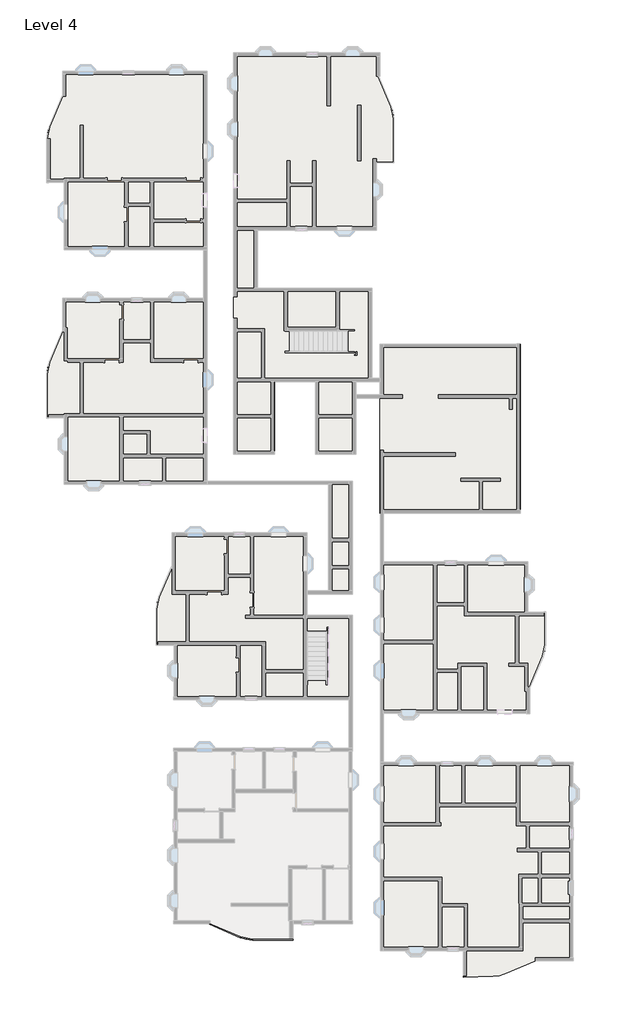
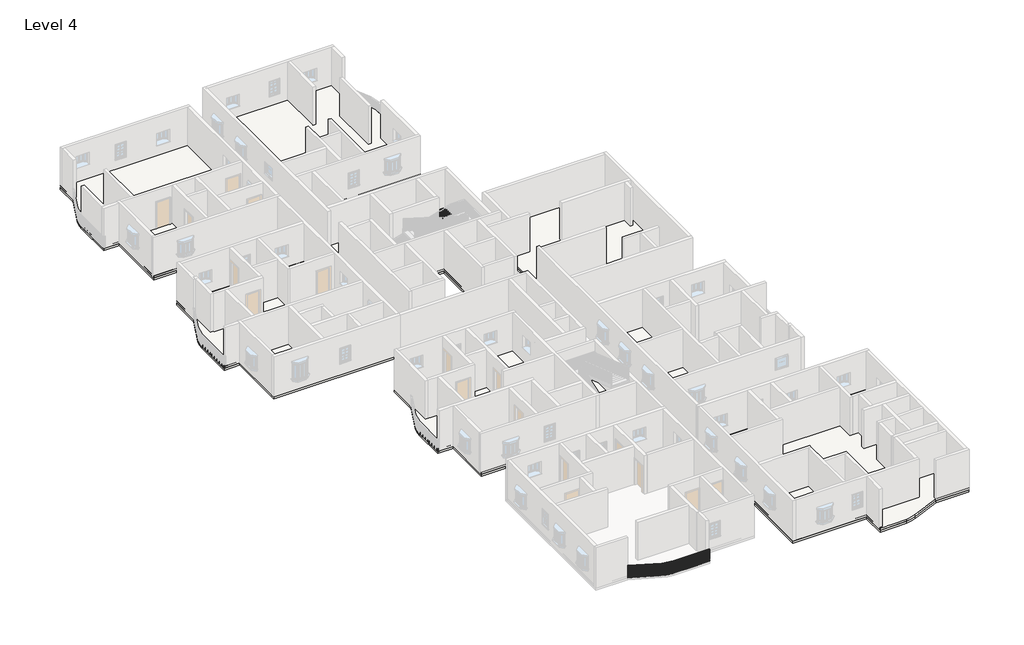
# One storey, part 5 of 14: 13 roofs, 12 slabs, 1 railing.
"""IFC4 building model written with IfcOpenShell, lengths in millimetres."""

from ifc_helpers import new_model, si_unit, point, frame, frame_2d, origin, place, context, project, spatial, polyline, circle_curve, trimmed, segment, composite_curve, outline, extrude, element, save
from ifc_brep_helpers import plane_surface, cylinder_surface, revolved_surface, advanced_brep

model = new_model("IFC4")

# Units and contexts
model_context = context("Model", 3, world=origin())
ifc_project = project(units=[si_unit("LENGTHUNIT", "METRE", prefix="MILLI")], contexts=[model_context])

# Site, building, storey
site = spatial("IfcSite", under=ifc_project)
building = spatial("IfcBuilding", under=site)
storey = spatial("IfcBuildingStorey", under=building, Name="Level 4", Elevation=9144.0)

# Railing
placement = place(None, origin())
element("IfcRailing", 1, ObjectType="Handrail - Rectangular", at=placement, inside=storey, context=model_context, shape_type="SolidModel", body=[
    advanced_brep(
    [(-10014.8722294, -25076.9923935, 10058.4), (-10014.8722294, -25076.9923935, 10007.6), (-10034.8694485, -25123.6909077, 10007.6), (-10034.8694485, -25123.6909077, 10058.4), (-8065.5370278, -25911.7359335, 10058.4), (-8065.5370278, -25911.7359335, 10007.6), (-8085.5342469, -25958.4344477, 10007.6), (-8085.5342469, -25958.4344477, 10058.4), (-7315.6413127, -26065.5416506, 10007.6), (-7315.6413127, -26065.5416506, 10058.4), (-7315.6413127, -26116.3416506, 10007.6), (-7315.6413127, -26116.3416506, 10058.4), (-4746.0891351, -26065.5416506, 10058.4), (-4746.0891351, -26116.3416506, 10058.4), (-4746.0891351, -26116.3416506, 10007.6), (-4746.0891351, -26065.5416506, 10007.6)],
    [
        (0, 1),
        (1, 2),
        (2, 3),
        (3, 0),
        (0, 4),
        (4, 5),
        (5, 1),
        (5, 6),
        (6, 2),
        (6, 7),
        (7, 3),
        (7, 4),
        (8, 5, circle_curve(frame((-7315.6413127, -24160.5416506, 10007.6), z_axis=(0.0, 0.0, -1.0), x_axis=(-0.3936460446736572, -0.9192620907623599, 0.0)), 1905.0)),
        (4, 9, circle_curve(frame((-7315.6413127, -24160.5416506, 10058.4), z_axis=(0.0, 0.0, 1.0), x_axis=(-0.3936460446736572, -0.9192620907623599, 0.0)), 1905.0)),
        (9, 8),
        (10, 6, circle_curve(frame((-7315.6413127, -24160.5416506, 10007.6), z_axis=(0.0, 0.0, -1.0), x_axis=(-0.3936460446736572, -0.9192620907623599, 0.0)), 1955.8)),
        (8, 10),
        (11, 7, circle_curve(frame((-7315.6413127, -24160.5416506, 10058.4), z_axis=(0.0, 0.0, -1.0), x_axis=(-0.3936460446736572, -0.9192620907623599, 0.0)), 1955.8)),
        (10, 11),
        (11, 9),
        (12, 13),
        (13, 14),
        (14, 15),
        (15, 12),
        (9, 12),
        (15, 8),
        (14, 10),
        (13, 11),
    ],
    [
        plane_surface(frame((-10024.8708389, -25100.3416506, 10058.4), z_axis=(-0.9192620907623597, 0.39364604467365766, 0.0), x_axis=(0.39364604467365766, 0.9192620907623597, 0.0))),
        plane_surface(frame((-10014.8722294, -25076.9923935, 10058.4), z_axis=(0.3936460446736573, 0.9192620907623599, 0.0), x_axis=(0.9192620907623599, -0.3936460446736573, 0.0))),
        plane_surface(frame((-10014.8722294, -25076.9923935, 10007.6), z_axis=(0.0, 0.0, -1.0000000000000002), x_axis=(0.9192620907623599, -0.3936460446736573, 0.0))),
        plane_surface(frame((-10034.8694485, -25123.6909077, 10007.6), z_axis=(-0.39364604467365766, -0.9192620907623597, 0.0), x_axis=(0.9192620907623597, -0.39364604467365766, 0.0))),
        plane_surface(frame((-10034.8694485, -25123.6909077, 10058.4), z_axis=(0.0, 0.0, 1.0), x_axis=(0.9192620907623597, -0.39364604467365766, 0.0))),
        revolved_surface(polyline([(-8065.537027803317, -25911.735933502296, 10058.4), (-8065.537027803317, -25911.735933502296, 10007.6)]), (-7315.6413127, -24160.5416506, 10058.4), (0.0, 0.0, 1.0)),
        plane_surface(frame((-7315.6413127, -24160.5416506, 10007.6), z_axis=(0.0, 0.0, -1.0), x_axis=(-0.3936460446736572, -0.9192620907623599, 0.0))),
        cylinder_surface(frame((-7315.6413127, -24160.5416506, 10058.4), z_axis=(0.0, 0.0, 1.0), x_axis=(-0.3936460446736572, -0.9192620907623599, 0.0)), 1955.8),
        plane_surface(frame((-7315.6413127, -24160.5416506, 10058.4), z_axis=(0.0, 0.0, 1.0), x_axis=(-0.3936460446736572, -0.9192620907623599, 0.0))),
        plane_surface(frame((-4746.0891351, -26090.9416506, 10058.4), z_axis=(1.0, 0.0, 0.0), x_axis=(0.0, 1.0, 0.0))),
        plane_surface(frame((-7315.6413127, -26065.5416506, 10058.4), z_axis=(0.0, 1.0, 0.0), x_axis=(1.0, 0.0, 0.0))),
        plane_surface(frame((-7315.6413127, -26065.5416506, 10007.6), z_axis=(0.0, 0.0, -1.0), x_axis=(1.0, 0.0, 0.0))),
        plane_surface(frame((-7315.6413127, -26116.3416506, 10007.6), z_axis=(0.0, -1.0, 0.0), x_axis=(1.0, 0.0, 0.0))),
        plane_surface(frame((-7315.6413127, -26116.3416506, 10058.4), z_axis=(0.0, 0.0, 1.0), x_axis=(1.0, 0.0, 0.0))),
    ],
    [
        (0, [[1, 2, 3, 4]]),
        (1, [[-1, 5, 6, 7]]),
        (2, [[-2, -7, 8, 9]]),
        (3, [[-3, -9, 10, 11]]),
        (4, [[-4, -11, 12, -5]]),
        (5, [[13, -6, 14, 15]]),
        (6, [[16, -8, -13, 17]]),
        (7, [[18, -10, -16, 19]]),
        (8, [[-14, -12, -18, 20]]),
        (9, [[21, 22, 23, 24]]),
        (10, [[-15, 25, -24, 26]]),
        (11, [[-17, -26, -23, 27]]),
        (12, [[-19, -27, -22, 28]]),
        (13, [[-20, -28, -21, -25]]),
    ],
),
    extrude(outline(polyline([(-4785.1663127, -26100.4666506), (-4785.1663127, -26081.4166506), (-4766.1163127, -26081.4166506), (-4766.1163127, -26100.4666506), (-4785.1663127, -26100.4666506)])), frame((0.0, 0.0, 9144.0), z_axis=(0.0, 0.0, 1.0), x_axis=(1.0, 0.0, 0.0)), (0.0, 0.0, 1.0), 863.6),
    extrude(outline(polyline([(-4886.7663127, -26100.4666506), (-4886.7663127, -26081.4166506), (-4867.7163127, -26081.4166506), (-4867.7163127, -26100.4666506), (-4886.7663127, -26100.4666506)])), frame((0.0, 0.0, 9144.0), z_axis=(0.0, 0.0, 1.0), x_axis=(1.0, 0.0, 0.0)), (0.0, 0.0, 1.0), 863.6),
    extrude(outline(polyline([(-4988.3663127, -26100.4666506), (-4988.3663127, -26081.4166506), (-4969.3163127, -26081.4166506), (-4969.3163127, -26100.4666506), (-4988.3663127, -26100.4666506)])), frame((0.0, 0.0, 9144.0), z_axis=(0.0, 0.0, 1.0), x_axis=(1.0, 0.0, 0.0)), (0.0, 0.0, 1.0), 863.6),
    extrude(outline(polyline([(-5089.9663127, -26100.4666506), (-5089.9663127, -26081.4166506), (-5070.9163127, -26081.4166506), (-5070.9163127, -26100.4666506), (-5089.9663127, -26100.4666506)])), frame((0.0, 0.0, 9144.0), z_axis=(0.0, 0.0, 1.0), x_axis=(1.0, 0.0, 0.0)), (0.0, 0.0, 1.0), 863.6),
    extrude(outline(polyline([(-5191.5663127, -26100.4666506), (-5191.5663127, -26081.4166506), (-5172.5163127, -26081.4166506), (-5172.5163127, -26100.4666506), (-5191.5663127, -26100.4666506)])), frame((0.0, 0.0, 9144.0), z_axis=(0.0, 0.0, 1.0), x_axis=(1.0, 0.0, 0.0)), (0.0, 0.0, 1.0), 863.6),
    extrude(outline(polyline([(-5293.1663127, -26100.4666506), (-5293.1663127, -26081.4166506), (-5274.1163127, -26081.4166506), (-5274.1163127, -26100.4666506), (-5293.1663127, -26100.4666506)])), frame((0.0, 0.0, 9144.0), z_axis=(0.0, 0.0, 1.0), x_axis=(1.0, 0.0, 0.0)), (0.0, 0.0, 1.0), 863.6),
    extrude(outline(polyline([(-5394.7663127, -26100.4666506), (-5394.7663127, -26081.4166506), (-5375.7163127, -26081.4166506), (-5375.7163127, -26100.4666506), (-5394.7663127, -26100.4666506)])), frame((0.0, 0.0, 9144.0), z_axis=(0.0, 0.0, 1.0), x_axis=(1.0, 0.0, 0.0)), (0.0, 0.0, 1.0), 863.6),
    extrude(outline(polyline([(-5496.3663127, -26100.4666506), (-5496.3663127, -26081.4166506), (-5477.3163127, -26081.4166506), (-5477.3163127, -26100.4666506), (-5496.3663127, -26100.4666506)])), frame((0.0, 0.0, 9144.0), z_axis=(0.0, 0.0, 1.0), x_axis=(1.0, 0.0, 0.0)), (0.0, 0.0, 1.0), 863.6),
    extrude(outline(polyline([(-5597.9663127, -26100.4666506), (-5597.9663127, -26081.4166506), (-5578.9163127, -26081.4166506), (-5578.9163127, -26100.4666506), (-5597.9663127, -26100.4666506)])), frame((0.0, 0.0, 9144.0), z_axis=(0.0, 0.0, 1.0), x_axis=(1.0, 0.0, 0.0)), (0.0, 0.0, 1.0), 863.6),
    extrude(outline(polyline([(-5699.5663127, -26100.4666506), (-5699.5663127, -26081.4166506), (-5680.5163127, -26081.4166506), (-5680.5163127, -26100.4666506), (-5699.5663127, -26100.4666506)])), frame((0.0, 0.0, 9144.0), z_axis=(0.0, 0.0, 1.0), x_axis=(1.0, 0.0, 0.0)), (0.0, 0.0, 1.0), 863.6),
    extrude(outline(polyline([(-5801.1663127, -26100.4666506), (-5801.1663127, -26081.4166506), (-5782.1163127, -26081.4166506), (-5782.1163127, -26100.4666506), (-5801.1663127, -26100.4666506)])), frame((0.0, 0.0, 9144.0), z_axis=(0.0, 0.0, 1.0), x_axis=(1.0, 0.0, 0.0)), (0.0, 0.0, 1.0), 863.6),
    extrude(outline(polyline([(-5902.7663127, -26100.4666506), (-5902.7663127, -26081.4166506), (-5883.7163127, -26081.4166506), (-5883.7163127, -26100.4666506), (-5902.7663127, -26100.4666506)])), frame((0.0, 0.0, 9144.0), z_axis=(0.0, 0.0, 1.0), x_axis=(1.0, 0.0, 0.0)), (0.0, 0.0, 1.0), 863.6),
    extrude(outline(polyline([(-6004.3663127, -26100.4666506), (-6004.3663127, -26081.4166506), (-5985.3163127, -26081.4166506), (-5985.3163127, -26100.4666506), (-6004.3663127, -26100.4666506)])), frame((0.0, 0.0, 9144.0), z_axis=(0.0, 0.0, 1.0), x_axis=(1.0, 0.0, 0.0)), (0.0, 0.0, 1.0), 863.6),
    extrude(outline(polyline([(-6105.9663127, -26100.4666506), (-6105.9663127, -26081.4166506), (-6086.9163127, -26081.4166506), (-6086.9163127, -26100.4666506), (-6105.9663127, -26100.4666506)])), frame((0.0, 0.0, 9144.0), z_axis=(0.0, 0.0, 1.0), x_axis=(1.0, 0.0, 0.0)), (0.0, 0.0, 1.0), 863.6),
    extrude(outline(polyline([(-6207.5663127, -26100.4666506), (-6207.5663127, -26081.4166506), (-6188.5163127, -26081.4166506), (-6188.5163127, -26100.4666506), (-6207.5663127, -26100.4666506)])), frame((0.0, 0.0, 9144.0), z_axis=(0.0, 0.0, 1.0), x_axis=(1.0, 0.0, 0.0)), (0.0, 0.0, 1.0), 863.6),
    extrude(outline(polyline([(-6309.1663127, -26100.4666506), (-6309.1663127, -26081.4166506), (-6290.1163127, -26081.4166506), (-6290.1163127, -26100.4666506), (-6309.1663127, -26100.4666506)])), frame((0.0, 0.0, 9144.0), z_axis=(0.0, 0.0, 1.0), x_axis=(1.0, 0.0, 0.0)), (0.0, 0.0, 1.0), 863.6),
    extrude(outline(polyline([(-6410.7663127, -26100.4666506), (-6410.7663127, -26081.4166506), (-6391.7163127, -26081.4166506), (-6391.7163127, -26100.4666506), (-6410.7663127, -26100.4666506)])), frame((0.0, 0.0, 9144.0), z_axis=(0.0, 0.0, 1.0), x_axis=(1.0, 0.0, 0.0)), (0.0, 0.0, 1.0), 863.6),
    extrude(outline(polyline([(-6512.3663127, -26100.4666506), (-6512.3663127, -26081.4166506), (-6493.3163127, -26081.4166506), (-6493.3163127, -26100.4666506), (-6512.3663127, -26100.4666506)])), frame((0.0, 0.0, 9144.0), z_axis=(0.0, 0.0, 1.0), x_axis=(1.0, 0.0, 0.0)), (0.0, 0.0, 1.0), 863.6),
    extrude(outline(polyline([(-6613.9663127, -26100.4666506), (-6613.9663127, -26081.4166506), (-6594.9163127, -26081.4166506), (-6594.9163127, -26100.4666506), (-6613.9663127, -26100.4666506)])), frame((0.0, 0.0, 9144.0), z_axis=(0.0, 0.0, 1.0), x_axis=(1.0, 0.0, 0.0)), (0.0, 0.0, 1.0), 863.6),
    extrude(outline(polyline([(-6715.5663127, -26100.4666506), (-6715.5663127, -26081.4166506), (-6696.5163127, -26081.4166506), (-6696.5163127, -26100.4666506), (-6715.5663127, -26100.4666506)])), frame((0.0, 0.0, 9144.0), z_axis=(0.0, 0.0, 1.0), x_axis=(1.0, 0.0, 0.0)), (0.0, 0.0, 1.0), 863.6),
    extrude(outline(polyline([(-6817.1663127, -26100.4666506), (-6817.1663127, -26081.4166506), (-6798.1163127, -26081.4166506), (-6798.1163127, -26100.4666506), (-6817.1663127, -26100.4666506)])), frame((0.0, 0.0, 9144.0), z_axis=(0.0, 0.0, 1.0), x_axis=(1.0, 0.0, 0.0)), (0.0, 0.0, 1.0), 863.6),
    extrude(outline(polyline([(-6918.7663127, -26100.4666506), (-6918.7663127, -26081.4166506), (-6899.7163127, -26081.4166506), (-6899.7163127, -26100.4666506), (-6918.7663127, -26100.4666506)])), frame((0.0, 0.0, 9144.0), z_axis=(0.0, 0.0, 1.0), x_axis=(1.0, 0.0, 0.0)), (0.0, 0.0, 1.0), 863.6),
    extrude(outline(polyline([(-7020.3663127, -26100.4666506), (-7020.3663127, -26081.4166506), (-7001.3163127, -26081.4166506), (-7001.3163127, -26100.4666506), (-7020.3663127, -26100.4666506)])), frame((0.0, 0.0, 9144.0), z_axis=(0.0, 0.0, 1.0), x_axis=(1.0, 0.0, 0.0)), (0.0, 0.0, 1.0), 863.6),
    extrude(outline(polyline([(-7121.9663127, -26100.4666506), (-7121.9663127, -26081.4166506), (-7102.9163127, -26081.4166506), (-7102.9163127, -26100.4666506), (-7121.9663127, -26100.4666506)])), frame((0.0, 0.0, 9144.0), z_axis=(0.0, 0.0, 1.0), x_axis=(1.0, 0.0, 0.0)), (0.0, 0.0, 1.0), 863.6),
    extrude(outline(polyline([(-7223.5663127, -26100.4666506), (-7223.5663127, -26081.4166506), (-7204.5163127, -26081.4166506), (-7204.5163127, -26100.4666506), (-7223.5663127, -26100.4666506)])), frame((0.0, 0.0, 9144.0), z_axis=(0.0, 0.0, 1.0), x_axis=(1.0, 0.0, 0.0)), (0.0, 0.0, 1.0), 863.6),
    extrude(outline(polyline([(-7395.3185803, -26098.8530973), (-7394.6296262, -26079.8155596), (-7375.5920885, -26080.5045137), (-7376.2810426, -26099.5420514), (-7395.3185803, -26098.8530973)])), frame((0.0, 0.0, 9144.0), z_axis=(0.0, 0.0, 1.0), x_axis=(1.0, 0.0, 0.0)), (0.0, 0.0, 1.0), 863.6),
    extrude(outline(polyline([(-7497.177549, -26091.9774704), (-7495.4880357, -26073.0025384), (-7476.5131037, -26074.6920517), (-7478.2026169, -26093.6669837), (-7497.177549, -26091.9774704)])), frame((0.0, 0.0, 9144.0), z_axis=(0.0, 0.0, 1.0), x_axis=(1.0, 0.0, 0.0)), (0.0, 0.0, 1.0), 863.6),
    extrude(outline(polyline([(-7598.5337632, -26079.7528408), (-7595.8483698, -26060.8930645), (-7576.9885935, -26063.5784579), (-7579.6739869, -26082.4382342), (-7598.5337632, -26079.7528408)])), frame((0.0, 0.0, 9144.0), z_axis=(0.0, 0.0, 1.0), x_axis=(1.0, 0.0, 0.0)), (0.0, 0.0, 1.0), 863.6),
    extrude(outline(polyline([(-7699.1065227, -26062.2130639), (-7695.4326862, -26043.5206744), (-7676.7402967, -26047.1945108), (-7680.4141332, -26065.8869003), (-7699.1065227, -26062.2130639)])), frame((0.0, 0.0, 9144.0), z_axis=(0.0, 0.0, 1.0), x_axis=(1.0, 0.0, 0.0)), (0.0, 0.0, 1.0), 863.6),
    extrude(outline(polyline([(-7798.6172969, -26039.4067149), (-7793.9651918, -26020.9334797), (-7775.4919566, -26025.5855848), (-7780.1440617, -26044.05882), (-7798.6172969, -26039.4067149)])), frame((0.0, 0.0, 9144.0), z_axis=(0.0, 0.0, 1.0), x_axis=(1.0, 0.0, 0.0)), (0.0, 0.0, 1.0), 863.6),
    extrude(outline(polyline([(-7896.7904963, -26011.396955), (-7891.1730064, -25993.1940347), (-7872.9700861, -25998.8115246), (-7878.587576, -26017.0144449), (-7896.7904963, -26011.396955)])), frame((0.0, 0.0, 9144.0), z_axis=(0.0, 0.0, 1.0), x_axis=(1.0, 0.0, 0.0)), (0.0, 0.0, 1.0), 863.6),
    extrude(outline(polyline([(-7993.3542357, -25978.2613554), (-7986.7869183, -25960.379162), (-7968.9047249, -25966.9464794), (-7975.4720423, -25984.8286729), (-7993.3542357, -25978.2613554)])), frame((0.0, 0.0, 9144.0), z_axis=(0.0, 0.0, 1.0), x_axis=(1.0, 0.0, 0.0)), (0.0, 0.0, 1.0), 863.6),
    extrude(outline(polyline([(-8169.4357205, -25905.2369062), (-8161.9367633, -25887.7249634), (-8144.4248205, -25895.2239205), (-8151.9237777, -25912.7358634), (-8169.4357205, -25905.2369062)])), frame((0.0, 0.0, 9144.0), z_axis=(0.0, 0.0, 1.0), x_axis=(1.0, 0.0, 0.0)), (0.0, 0.0, 1.0), 863.6),
    extrude(outline(polyline([(-8262.8327489, -25865.2424681), (-8255.3337918, -25847.7305252), (-8237.8218489, -25855.2294824), (-8245.3208061, -25872.7414252), (-8262.8327489, -25865.2424681)])), frame((0.0, 0.0, 9144.0), z_axis=(0.0, 0.0, 1.0), x_axis=(1.0, 0.0, 0.0)), (0.0, 0.0, 1.0), 863.6),
    extrude(outline(polyline([(-8356.2297773, -25825.2480299), (-8348.7308202, -25807.7360871), (-8331.2188774, -25815.2350443), (-8338.7178345, -25832.7469871), (-8356.2297773, -25825.2480299)])), frame((0.0, 0.0, 9144.0), z_axis=(0.0, 0.0, 1.0), x_axis=(1.0, 0.0, 0.0)), (0.0, 0.0, 1.0), 863.6),
    extrude(outline(polyline([(-8449.6268058, -25785.2535918), (-8442.1278486, -25767.741649), (-8424.6159058, -25775.2406061), (-8432.1148629, -25792.752549), (-8449.6268058, -25785.2535918)])), frame((0.0, 0.0, 9144.0), z_axis=(0.0, 0.0, 1.0), x_axis=(1.0, 0.0, 0.0)), (0.0, 0.0, 1.0), 863.6),
    extrude(outline(polyline([(-8543.0238342, -25745.2591537), (-8535.524877, -25727.7472108), (-8518.0129342, -25735.246168), (-8525.5118914, -25752.7581108), (-8543.0238342, -25745.2591537)])), frame((0.0, 0.0, 9144.0), z_axis=(0.0, 0.0, 1.0), x_axis=(1.0, 0.0, 0.0)), (0.0, 0.0, 1.0), 863.6),
    extrude(outline(polyline([(-8636.4208626, -25705.2647155), (-8628.9219055, -25687.7527727), (-8611.4099626, -25695.2517298), (-8618.9089198, -25712.7636727), (-8636.4208626, -25705.2647155)])), frame((0.0, 0.0, 9144.0), z_axis=(0.0, 0.0, 1.0), x_axis=(1.0, 0.0, 0.0)), (0.0, 0.0, 1.0), 863.6),
    extrude(outline(polyline([(-8729.817891, -25665.2702774), (-8722.3189339, -25647.7583346), (-8704.806991, -25655.2572917), (-8712.3059482, -25672.7692345), (-8729.817891, -25665.2702774)])), frame((0.0, 0.0, 9144.0), z_axis=(0.0, 0.0, 1.0), x_axis=(1.0, 0.0, 0.0)), (0.0, 0.0, 1.0), 863.6),
    extrude(outline(polyline([(-8823.2149194, -25625.2758392), (-8815.7159623, -25607.7638964), (-8798.2040195, -25615.2628536), (-8805.7029766, -25632.7747964), (-8823.2149194, -25625.2758392)])), frame((0.0, 0.0, 9144.0), z_axis=(0.0, 0.0, 1.0), x_axis=(1.0, 0.0, 0.0)), (0.0, 0.0, 1.0), 863.6),
    extrude(outline(polyline([(-8916.6119479, -25585.2814011), (-8909.1129907, -25567.7694583), (-8891.6010479, -25575.2684154), (-8899.100005, -25592.7803583), (-8916.6119479, -25585.2814011)])), frame((0.0, 0.0, 9144.0), z_axis=(0.0, 0.0, 1.0), x_axis=(1.0, 0.0, 0.0)), (0.0, 0.0, 1.0), 863.6),
    extrude(outline(polyline([(-9010.0089763, -25545.286963), (-9002.5100191, -25527.7750201), (-8984.9980763, -25535.2739773), (-8992.4970335, -25552.7859201), (-9010.0089763, -25545.286963)])), frame((0.0, 0.0, 9144.0), z_axis=(0.0, 0.0, 1.0), x_axis=(1.0, 0.0, 0.0)), (0.0, 0.0, 1.0), 863.6),
    extrude(outline(polyline([(-9103.4060047, -25505.2925248), (-9095.9070476, -25487.780582), (-9078.3951047, -25495.2795391), (-9085.8940619, -25512.791482), (-9103.4060047, -25505.2925248)])), frame((0.0, 0.0, 9144.0), z_axis=(0.0, 0.0, 1.0), x_axis=(1.0, 0.0, 0.0)), (0.0, 0.0, 1.0), 863.6),
    extrude(outline(polyline([(-9196.8030331, -25465.2980867), (-9189.304076, -25447.7861439), (-9171.7921332, -25455.285101), (-9179.2910903, -25472.7970438), (-9196.8030331, -25465.2980867)])), frame((0.0, 0.0, 9144.0), z_axis=(0.0, 0.0, 1.0), x_axis=(1.0, 0.0, 0.0)), (0.0, 0.0, 1.0), 863.6),
    extrude(outline(polyline([(-9290.2000616, -25425.3036485), (-9282.7011044, -25407.7917057), (-9265.1891616, -25415.2906629), (-9272.6881187, -25432.8026057), (-9290.2000616, -25425.3036485)])), frame((0.0, 0.0, 9144.0), z_axis=(0.0, 0.0, 1.0), x_axis=(1.0, 0.0, 0.0)), (0.0, 0.0, 1.0), 863.6),
    extrude(outline(polyline([(-9383.59709, -25385.3092104), (-9376.0981328, -25367.7972676), (-9358.58619, -25375.2962247), (-9366.0851471, -25392.8081676), (-9383.59709, -25385.3092104)])), frame((0.0, 0.0, 9144.0), z_axis=(0.0, 0.0, 1.0), x_axis=(1.0, 0.0, 0.0)), (0.0, 0.0, 1.0), 863.6),
    extrude(outline(polyline([(-9476.9941184, -25345.3147723), (-9469.4951612, -25327.8028294), (-9451.9832184, -25335.3017866), (-9459.4821756, -25352.8137294), (-9476.9941184, -25345.3147723)])), frame((0.0, 0.0, 9144.0), z_axis=(0.0, 0.0, 1.0), x_axis=(1.0, 0.0, 0.0)), (0.0, 0.0, 1.0), 863.6),
    extrude(outline(polyline([(-9570.3911468, -25305.3203341), (-9562.8921897, -25287.8083913), (-9545.3802468, -25295.3073485), (-9552.879204, -25312.8192913), (-9570.3911468, -25305.3203341)])), frame((0.0, 0.0, 9144.0), z_axis=(0.0, 0.0, 1.0), x_axis=(1.0, 0.0, 0.0)), (0.0, 0.0, 1.0), 863.6),
    extrude(outline(polyline([(-9663.7881752, -25265.325896), (-9656.2892181, -25247.8139532), (-9638.7772753, -25255.3129103), (-9646.2762324, -25272.8248531), (-9663.7881752, -25265.325896)])), frame((0.0, 0.0, 9144.0), z_axis=(0.0, 0.0, 1.0), x_axis=(1.0, 0.0, 0.0)), (0.0, 0.0, 1.0), 863.6),
    extrude(outline(polyline([(-9757.1852037, -25225.3314579), (-9749.6862465, -25207.819515), (-9732.1743037, -25215.3184722), (-9739.6732608, -25232.830415), (-9757.1852037, -25225.3314579)])), frame((0.0, 0.0, 9144.0), z_axis=(0.0, 0.0, 1.0), x_axis=(1.0, 0.0, 0.0)), (0.0, 0.0, 1.0), 863.6),
    extrude(outline(polyline([(-9850.5822321, -25185.3370197), (-9843.0832749, -25167.8250769), (-9825.5713321, -25175.324034), (-9833.0702893, -25192.8359769), (-9850.5822321, -25185.3370197)])), frame((0.0, 0.0, 9144.0), z_axis=(0.0, 0.0, 1.0), x_axis=(1.0, 0.0, 0.0)), (0.0, 0.0, 1.0), 863.6),
    extrude(outline(polyline([(-9943.9792605, -25145.3425816), (-9936.4803034, -25127.8306387), (-9918.9683605, -25135.3295959), (-9926.4673177, -25152.8415387), (-9943.9792605, -25145.3425816)])), frame((0.0, 0.0, 9144.0), z_axis=(0.0, 0.0, 1.0), x_axis=(1.0, 0.0, 0.0)), (0.0, 0.0, 1.0), 863.6),
    extrude(outline(polyline([(-7325.1663127, -26100.4666506), (-7325.1663127, -26081.4166506), (-7306.1163127, -26081.4166506), (-7306.1163127, -26100.4666506), (-7325.1663127, -26100.4666506)])), frame((0.0, 0.0, 9144.0), z_axis=(0.0, 0.0, 1.0), x_axis=(1.0, 0.0, 0.0)), (0.0, 0.0, 1.0), 863.6),
    extrude(outline(polyline([(-8088.0410874, -25940.0916834), (-8080.5421302, -25922.5797406), (-8063.0301874, -25930.0786978), (-8070.5291445, -25947.5906406), (-8088.0410874, -25940.0916834)])), frame((0.0, 0.0, 9144.0), z_axis=(0.0, 0.0, 1.0), x_axis=(1.0, 0.0, 0.0)), (0.0, 0.0, 1.0), 863.6),
    extrude(outline(polyline([(-4765.1391351, -26100.4666506), (-4765.1391351, -26081.4166506), (-4746.0891351, -26081.4166506), (-4746.0891351, -26100.4666506), (-4765.1391351, -26100.4666506)])), frame((0.0, 0.0, 9144.0), z_axis=(0.0, 0.0, 1.0), x_axis=(1.0, 0.0, 0.0)), (0.0, 0.0, 1.0), 863.6),
    extrude(outline(polyline([(-10028.6203175, -25109.097622), (-10021.1213604, -25091.5856792), (-10003.6094175, -25099.0846363), (-10011.1083747, -25116.5965792), (-10028.6203175, -25109.097622)])), frame((0.0, 0.0, 9144.0), z_axis=(0.0, 0.0, 1.0), x_axis=(1.0, 0.0, 0.0)), (0.0, 0.0, 1.0), 863.6),
])

# Roofs
element("IfcRoof", 2, ObjectType="Generic - 12\"", at=placement, inside=storey, context=model_context, shape_type="SweptSolid", body=[
    extrude(outline(composite_curve([segment(polyline([(6070.4380523, -26783.9042694), (812.6380523, -26783.9042694), (812.6380523, -14845.9042694), (13017.3380523, -14845.9042694), (13017.3380523, -27431.6042694), (10660.5280667, -27431.6042694), (8711.1928652, -28266.3478094)]), True, "CONTINUOUS"), segment(trimmed(circle_curve(frame_2d((7951.2985405, -26491.8042694)), 1930.4), [point((8711.1928652, -28266.3478094))], [point((7953.0959373, -28422.2034326))], False, "CARTESIAN"), True, "CONTINUOUS"), segment(polyline([(7953.0959373, -28422.2034326), (6070.4380523, -28487.9472947), (6070.4380523, -26783.9042694)]), True, "CONTINUOUS")], self_intersect=False)), frame((0.0, 0.0, 9144.0), z_axis=(0.0, 0.0, 1.0), x_axis=(1.0, 0.0, 0.0)), (0.0, 0.0, 1.0), 152.4),
])
element("IfcRoof", 3, ObjectType="Generic - 12\"", at=placement, inside=storey, context=model_context, shape_type="SweptSolid", body=[
    extrude(outline(composite_curve([segment(polyline([(10274.1380523, -11759.8042694), (803.8108649, -11759.8042694), (803.8108649, -2133.2042694), (10159.8380523, -2133.2042694), (10159.8380523, -5352.6542694), (11264.7380523, -5352.6542694), (11264.7380523, -7397.5810633)]), True, "CONTINUOUS"), segment(trimmed(circle_curve(frame_2d((9334.3380523, -7397.5810633)), 1930.4), [point((11264.7380523, -7397.5810633))], [point((11108.8815923, -8157.475388))], False, "CARTESIAN"), True, "CONTINUOUS"), segment(polyline([(11108.8815923, -8157.475388), (10274.1380523, -10106.8105895), (10274.1380523, -11759.8042694)]), True, "CONTINUOUS")], self_intersect=False)), frame((0.0, 0.0, 9144.0), z_axis=(0.0, 0.0, 1.0), x_axis=(1.0, 0.0, 0.0)), (0.0, 0.0, 1.0), 152.4),
])
element("IfcRoof", 4, ObjectType="Generic - 12\"", at=placement, inside=storey, context=model_context, shape_type="SweptSolid", body=[
    extrude(outline(composite_curve([segment(polyline([(-13395.387215, -7421.9416506), (-13395.387215, -5140.4900045)]), True, "CONTINUOUS"), segment(trimmed(circle_curve(frame_2d((-11464.987215, -5140.4900045)), 1930.4), [point((-13395.387215, -5140.4900045))], [point((-13239.530755, -4380.5956799))], False, "CARTESIAN"), True, "CONTINUOUS"), segment(polyline([(-13239.530755, -4380.5956799), (-12404.787215, -2431.2604783), (-12404.787215, -322.6416506), (-3857.687215, -322.6416506), (-3857.687215, -5523.2916506), (-974.1891351, -5523.2916506), (-974.1891351, -10889.0416506), (-12290.487215, -10889.0416506), (-12290.487215, -7421.9416506), (-13395.387215, -7421.9416506)]), True, "CONTINUOUS")], self_intersect=False)), frame((0.0, 0.0, 9144.0), z_axis=(0.0, 0.0, 1.0), x_axis=(1.0, 0.0, 0.0)), (0.0, 0.0, 1.0), 152.4),
])
element("IfcRoof", 5, ObjectType="Generic - 12\"", at=placement, inside=storey, context=model_context, shape_type="SweptSolid", body=[
    extrude(outline(polyline([(-2472.7891351, 2953.9583494), (-961.4891351, 2953.9583494), (-961.4891351, -4202.4916506), (-2472.7891351, -4202.4916506), (-2472.7891351, 2953.9583494)])), frame((0.0, 0.0, 9144.0), z_axis=(0.0, 0.0, 1.0), x_axis=(1.0, 0.0, 0.0)), (0.0, 0.0, 1.0), 152.4),
])
element("IfcRoof", 6, ObjectType="Generic - 12\"", at=placement, inside=storey, context=model_context, shape_type="SweptSolid", body=[
    extrude(outline(composite_curve([segment(polyline([(-10194.3891351, 2750.7583494), (-19236.7891351, 2750.7583494), (-19236.7891351, 6979.8583494), (-20341.6891351, 6979.8583494), (-20341.6891351, 9746.7948172)]), True, "CONTINUOUS"), segment(trimmed(circle_curve(frame_2d((-18411.2891351, 9746.7948172)), 1930.4), [point((-20341.6891351, 9746.7948172))], [point((-20185.8326751, 10506.6891419))], False, "CARTESIAN"), True, "CONTINUOUS"), segment(polyline([(-20185.8326751, 10506.6891419), (-19351.0891351, 12456.0243434), (-19351.0891351, 14536.3583494), (-10194.3891351, 14536.3583494), (-10194.3891351, 2750.7583494)]), True, "CONTINUOUS")], self_intersect=False)), frame((0.0, 0.0, 9144.0), z_axis=(0.0, 0.0, 1.0), x_axis=(1.0, 0.0, 0.0)), (0.0, 0.0, 1.0), 152.4),
])
element("IfcRoof", 7, ObjectType="Generic - 12\"", at=placement, inside=storey, context=model_context, shape_type="SweptSolid", body=[
    extrude(outline(composite_curve([segment(polyline([(-10194.3891351, 17609.7583494), (-19236.7891351, 17609.7583494), (-19236.7891351, 21889.6583494), (-20341.6891351, 21889.6583494), (-20341.6891351, 24656.5948172)]), True, "CONTINUOUS"), segment(trimmed(circle_curve(frame_2d((-18411.2891351, 24656.5948172)), 1930.4), [point((-20341.6891351, 24656.5948172))], [point((-20185.8326751, 25416.4891419))], False, "CARTESIAN"), True, "CONTINUOUS"), segment(polyline([(-20185.8326751, 25416.4891419), (-19351.0891351, 27365.8243434), (-19351.0891351, 28950.8583494), (-10194.3891351, 28950.8583494), (-10194.3891351, 17609.7583494)]), True, "CONTINUOUS")], self_intersect=False)), frame((0.0, 0.0, 9144.0), z_axis=(0.0, 0.0, 1.0), x_axis=(1.0, 0.0, 0.0)), (0.0, 0.0, 1.0), 152.4),
])
element("IfcRoof", 8, ObjectType="Generic - 12\"", at=placement, inside=storey, context=model_context, shape_type="SweptSolid", body=[
    extrude(outline(composite_curve([segment(polyline([(-8492.5891351, 18875.1215905), (-8492.5891351, 30101.9215905), (664.1108649, 30101.9215905), (664.1108649, 28631.1875845), (1498.8544049, 26681.8523829)]), True, "CONTINUOUS"), segment(trimmed(circle_curve(frame_2d((-275.6891351, 25921.9580583)), 1930.4), [point((1498.8544049, 26681.8523829))], [point((1654.7108649, 25921.9580583))], False, "CARTESIAN"), True, "CONTINUOUS"), segment(polyline([(1654.7108649, 25921.9580583), (1654.7108649, 23155.0215905), (549.8108649, 23155.0215905), (549.8108649, 18875.1215905), (-8492.5891351, 18875.1215905)]), True, "CONTINUOUS")], self_intersect=False)), frame((0.0, 0.0, 9144.0), z_axis=(0.0, 0.0, 1.0), x_axis=(1.0, 0.0, 0.0)), (0.0, 0.0, 1.0), 152.4),
])
element("IfcRoof", 9, ObjectType="Generic - 12\"", at=placement, inside=storey, context=model_context, shape_type="SweptSolid", body=[
    extrude(outline(polyline([(-8492.5891351, 9478.4949943), (-5914.4891351, 9478.4949943), (-5914.4891351, 4665.1949943), (-8492.5891351, 4665.1949943), (-8492.5891351, 9478.4949943)])), frame((0.0, 0.0, 9144.0), z_axis=(0.0, 0.0, 1.0), x_axis=(1.0, 0.0, 0.0)), (0.0, 0.0, 1.0), 152.4),
])
element("IfcRoof", 10, ObjectType="Generic - 12\"", at=placement, inside=storey, context=model_context, shape_type="SweptSolid", body=[
    extrude(outline(polyline([(-3310.9891351, 9478.4949943), (-745.5891351, 9478.4949943), (-745.5891351, 4652.4949943), (-3310.9891351, 4652.4949943), (-3310.9891351, 9478.4949943)])), frame((0.0, 0.0, 9144.0), z_axis=(0.0, 0.0, 1.0), x_axis=(1.0, 0.0, 0.0)), (0.0, 0.0, 1.0), 152.4),
])
element("IfcRoof", 11, ObjectType="Generic - 12\"", at=placement, inside=storey, context=model_context, shape_type="SweptSolid", body=[
    extrude(outline(polyline([(-8492.5891351, 19078.3215905), (-6993.9891351, 19078.3215905), (-6993.9891351, 14988.9215905), (-8492.5891351, 14988.9215905), (-8492.5891351, 19078.3215905)])), frame((0.0, 0.0, 9144.0), z_axis=(0.0, 0.0, 1.0), x_axis=(1.0, 0.0, 0.0)), (0.0, 0.0, 1.0), 152.4),
])
element("IfcRoof", 12, ObjectType="Generic - 12\"", at=placement, inside=storey, context=model_context, shape_type="SweptSolid", body=[
    extrude(outline(polyline([(-8492.5891351, 15192.1215905), (257.7108649, 15192.1215905), (257.7108649, 9275.2949943), (-8492.5891351, 9275.2949943), (-8492.5891351, 15192.1215905)])), frame((0.0, 0.0, 9144.0), z_axis=(0.0, 0.0, 1.0), x_axis=(1.0, 0.0, 0.0)), (0.0, 0.0, 1.0), 152.4),
])
element("IfcRoof", 13, ObjectType="Generic - 12\"", at=placement, inside=storey, context=model_context, shape_type="SweptSolid", body=[
    extrude(outline(polyline([(793.5880523, 11646.2957306), (9677.2380523, 11646.2957306), (9677.2380523, 940.1957306), (793.5880523, 940.1957306), (793.5880523, 11646.2957306)])), frame((0.0, 0.0, 9144.0), z_axis=(0.0, 0.0, 1.0), x_axis=(1.0, 0.0, 0.0)), (0.0, 0.0, 1.0), 152.4),
])
element("IfcRoof", 14, ObjectType="Generic - 12\"", at=placement, inside=storey, context=model_context, shape_type="SweptSolid", body=[
    extrude(outline(composite_curve([segment(polyline([(-8492.5891351, 18875.1215905), (-8492.5891351, 30101.9215905), (664.1108649, 30101.9215905), (664.1108649, 28631.1875845), (1498.8544049, 26681.8523829)]), True, "CONTINUOUS"), segment(trimmed(circle_curve(frame_2d((-275.6891351, 25921.9580583)), 1930.4), [point((1498.8544049, 26681.8523829))], [point((1654.7108649, 25921.9580583))], False, "CARTESIAN"), True, "CONTINUOUS"), segment(polyline([(1654.7108649, 25921.9580583), (1654.7108649, 23155.0215905), (549.8108649, 23155.0215905), (549.8108649, 18875.1215905), (-8492.5891351, 18875.1215905)]), True, "CONTINUOUS")], self_intersect=False)), frame((0.0, 0.0, 9144.0), z_axis=(0.0, 0.0, 1.0), x_axis=(1.0, 0.0, 0.0)), (0.0, 0.0, 1.0), 152.4),
])

# Slabs
element("IfcSlab", 15, ObjectType="Generic - 12\"", at=placement, inside=storey, context=model_context, shape_type="SweptSolid", body=[
    extrude(outline(composite_curve([segment(polyline([(-20341.6891351, 21889.6583494), (-20341.6891351, 24656.5948172)]), True, "CONTINUOUS"), segment(trimmed(circle_curve(frame_2d((-18411.2891351, 24656.5948172)), 1930.4), [point((-20341.6891351, 24656.5948172))], [point((-20185.8326751, 25416.4891419))], False, "CARTESIAN"), True, "CONTINUOUS"), segment(polyline([(-20185.8326751, 25416.4891419), (-19351.0891351, 27365.8243434), (-19351.0891351, 28950.8583494), (-10194.3891351, 28950.8583494), (-10194.3891351, 17609.7583494), (-19236.7891351, 17609.7583494), (-19236.7891351, 21889.6583494), (-20341.6891351, 21889.6583494)]), True, "CONTINUOUS")], self_intersect=False)), frame((0.0, 0.0, 8991.6), z_axis=(0.0, 0.0, 1.0), x_axis=(1.0, 0.0, 0.0)), (0.0, 0.0, 1.0), 152.4),
])
element("IfcSlab", 16, ObjectType="Generic - 12\"", at=placement, inside=storey, context=model_context, shape_type="SweptSolid", body=[
    extrude(outline(composite_curve([segment(polyline([(13017.3380523, -27431.6042694), (10660.5280667, -27431.6042694), (8711.1928652, -28266.3478094)]), True, "CONTINUOUS"), segment(trimmed(circle_curve(frame_2d((7951.2985405, -26491.8042694)), 1930.4), [point((8711.1928652, -28266.3478094))], [point((7953.0959373, -28422.2034326))], False, "CARTESIAN"), True, "CONTINUOUS"), segment(polyline([(7953.0959373, -28422.2034326), (6070.4380523, -28487.9472947), (6070.4380523, -26783.9042694), (812.6380523, -26783.9042694), (812.6380523, -14845.9042694), (13017.3380523, -14845.9042694), (13017.3380523, -27431.6042694)]), True, "CONTINUOUS")], self_intersect=False)), frame((0.0, 0.0, 8991.6), z_axis=(0.0, 0.0, 1.0), x_axis=(1.0, 0.0, 0.0)), (0.0, 0.0, 1.0), 152.4),
])
element("IfcSlab", 17, ObjectType="Generic - 12\"", at=placement, inside=storey, context=model_context, shape_type="SweptSolid", body=[
    extrude(outline(composite_curve([segment(polyline([(10274.1380523, -11759.8042694), (803.8108649, -11759.8042694), (803.8108649, -2133.2042694), (10159.8380523, -2133.2042694), (10159.8380523, -5352.6542694), (11264.7380523, -5352.6542694), (11264.7380523, -7397.5810633)]), True, "CONTINUOUS"), segment(trimmed(circle_curve(frame_2d((9334.3380523, -7397.5810633)), 1930.4), [point((11264.7380523, -7397.5810633))], [point((11108.8815923, -8157.475388))], False, "CARTESIAN"), True, "CONTINUOUS"), segment(polyline([(11108.8815923, -8157.475388), (10274.1380523, -10106.8105895), (10274.1380523, -11759.8042694)]), True, "CONTINUOUS")], self_intersect=False)), frame((0.0, 0.0, 8991.6), z_axis=(0.0, 0.0, 1.0), x_axis=(1.0, 0.0, 0.0)), (0.0, 0.0, 1.0), 152.4),
])
element("IfcSlab", 18, ObjectType="Generic - 12\"", at=placement, inside=storey, context=model_context, shape_type="SweptSolid", body=[
    extrude(outline(composite_curve([segment(polyline([(-974.1891351, -10889.0416506), (-12290.487215, -10889.0416506), (-12290.487215, -7421.9416506), (-13395.387215, -7421.9416506), (-13395.387215, -5140.4900045)]), True, "CONTINUOUS"), segment(trimmed(circle_curve(frame_2d((-11464.987215, -5140.4900045)), 1930.4), [point((-13395.387215, -5140.4900045))], [point((-13239.530755, -4380.5956799))], False, "CARTESIAN"), True, "CONTINUOUS"), segment(polyline([(-13239.530755, -4380.5956799), (-12404.787215, -2431.2604783), (-12404.787215, -322.6416506), (-3857.687215, -322.6416506), (-3857.687215, -5523.2916506), (-974.1891351, -5523.2916506), (-974.1891351, -10889.0416506)]), True, "CONTINUOUS")], self_intersect=False)), frame((0.0, 0.0, 8991.6), z_axis=(0.0, 0.0, 1.0), x_axis=(1.0, 0.0, 0.0)), (0.0, 0.0, 1.0), 152.4),
])
element("IfcSlab", 19, ObjectType="Generic - 12\"", at=placement, inside=storey, context=model_context, shape_type="SweptSolid", body=[
    extrude(outline(composite_curve([segment(polyline([(-20341.6891351, 6979.8583494), (-20341.6891351, 9746.7948172)]), True, "CONTINUOUS"), segment(trimmed(circle_curve(frame_2d((-18411.2891351, 9746.7948172)), 1930.4), [point((-20341.6891351, 9746.7948172))], [point((-20185.8326751, 10506.6891419))], False, "CARTESIAN"), True, "CONTINUOUS"), segment(polyline([(-20185.8326751, 10506.6891419), (-19351.0891351, 12456.0243434), (-19351.0891351, 14536.3583494), (-10194.3891351, 14536.3583494), (-10194.3891351, 2750.7583494), (-19236.7891351, 2750.7583494), (-19236.7891351, 6979.8583494), (-20341.6891351, 6979.8583494)]), True, "CONTINUOUS")], self_intersect=False)), frame((0.0, 0.0, 8991.6), z_axis=(0.0, 0.0, 1.0), x_axis=(1.0, 0.0, 0.0)), (0.0, 0.0, 1.0), 152.4),
])
element("IfcSlab", 20, ObjectType="Generic - 12\"", at=placement, inside=storey, context=model_context, shape_type="SweptSolid", body=[
    extrude(outline(composite_curve([segment(polyline([(549.8108649, 18875.1215905), (-8492.5891351, 18875.1215905), (-8492.5891351, 30101.9215905), (664.1108649, 30101.9215905), (664.1108649, 28631.1875845), (1498.8544049, 26681.8523829)]), True, "CONTINUOUS"), segment(trimmed(circle_curve(frame_2d((-275.6891351, 25921.9580583)), 1930.4), [point((1498.8544049, 26681.8523829))], [point((1654.7108649, 25921.9580583))], False, "CARTESIAN"), True, "CONTINUOUS"), segment(polyline([(1654.7108649, 25921.9580583), (1654.7108649, 23155.0215905), (549.8108649, 23155.0215905), (549.8108649, 18875.1215905)]), True, "CONTINUOUS")], self_intersect=False)), frame((0.0, 0.0, 8991.6), z_axis=(0.0, 0.0, 1.0), x_axis=(1.0, 0.0, 0.0)), (0.0, 0.0, 1.0), 152.4),
])
element("IfcSlab", 21, ObjectType="Generic - 12\"", at=placement, inside=storey, context=model_context, shape_type="SweptSolid", body=[
    extrude(outline(polyline([(257.7108649, 15192.1215905), (257.7108649, 9275.2949943), (-8492.5891351, 9275.2949943), (-8492.5891351, 15192.1215905), (257.7108649, 15192.1215905)])), frame((0.0, 0.0, 8991.6), z_axis=(0.0, 0.0, 1.0), x_axis=(1.0, 0.0, 0.0)), (0.0, 0.0, 1.0), 152.4),
])
element("IfcSlab", 22, ObjectType="Generic - 12\"", at=placement, inside=storey, context=model_context, shape_type="SweptSolid", body=[
    extrude(outline(polyline([(9677.2380523, 11646.2957306), (9677.2380523, 940.1957306), (793.5880523, 940.1957306), (793.5880523, 11646.2957306), (9677.2380523, 11646.2957306)])), frame((0.0, 0.0, 8991.6), z_axis=(0.0, 0.0, 1.0), x_axis=(1.0, 0.0, 0.0)), (0.0, 0.0, 1.0), 152.4),
])
element("IfcSlab", 23, ObjectType="Generic - 12\"", at=placement, inside=storey, context=model_context, shape_type="SweptSolid", body=[
    extrude(outline(polyline([(-5914.4891351, 9478.4949943), (-5914.4891351, 4665.1949943), (-8492.5891351, 4665.1949943), (-8492.5891351, 9478.4949943), (-5914.4891351, 9478.4949943)])), frame((0.0, 0.0, 8991.6), z_axis=(0.0, 0.0, 1.0), x_axis=(1.0, 0.0, 0.0)), (0.0, 0.0, 1.0), 152.4),
])
element("IfcSlab", 24, ObjectType="Generic - 12\"", at=placement, inside=storey, context=model_context, shape_type="SweptSolid", body=[
    extrude(outline(polyline([(-745.5891351, 9478.4949943), (-745.5891351, 4652.4949943), (-3310.9891351, 4652.4949943), (-3310.9891351, 9478.4949943), (-745.5891351, 9478.4949943)])), frame((0.0, 0.0, 8991.6), z_axis=(0.0, 0.0, 1.0), x_axis=(1.0, 0.0, 0.0)), (0.0, 0.0, 1.0), 152.4),
])
element("IfcSlab", 25, ObjectType="Generic - 12\"", at=placement, inside=storey, context=model_context, shape_type="SweptSolid", body=[
    extrude(outline(polyline([(-961.4891351, 2953.9583494), (-961.4891351, -4202.4916506), (-2472.7891351, -4202.4916506), (-2472.7891351, 2953.9583494), (-961.4891351, 2953.9583494)])), frame((0.0, 0.0, 8991.6), z_axis=(0.0, 0.0, 1.0), x_axis=(1.0, 0.0, 0.0)), (0.0, 0.0, 1.0), 152.4),
])
element("IfcSlab", 26, ObjectType="Generic - 12\"", at=placement, inside=storey, context=model_context, shape_type="SweptSolid", body=[
    extrude(outline(polyline([(-961.4891351, 2953.9583494), (-961.4891351, -4202.4916506), (-2472.7891351, -4202.4916506), (-2472.7891351, 2953.9583494), (-961.4891351, 2953.9583494)])), frame((0.0, 0.0, 8991.6), z_axis=(0.0, 0.0, 1.0), x_axis=(1.0, 0.0, 0.0)), (0.0, 0.0, 1.0), 152.4),
])

save(model, "model.ifc")

# Revit data of these elements
# Type "Handrail - Rectangular"
#   Assembly Code = "C2010400"
#   built-in parameter 1008612 = 0.0416667 (stored number, unit not read)
#   built-in parameter 1008611 = 0.0416667 (stored number, unit not read)
#   built-in parameter 1008609 = 0.333333 (stored number, unit not read)
#   built-in parameter 1008604 = 0.166667 (stored number, unit not read)
#   built-in parameter 1008603 = 0.166667 (stored number, unit not read)
#   Railing Height = 3' - 0"
#   built-in parameter 1008630 = 2
#   built-in parameter 1008610 = 2
#   built-in parameter 1008618 = Baluster - Square : 3/4"
# Type "Generic - 12\""
#   Assembly Code = "B1020"
#   Layers, outside or top first: 0' - 6" no material (function 1)
# Type "Generic - 12\""
#   Assembly Code = "B1010"
#   Function = 0
#   Layers, outside or top first: 0' - 6" no material (function 1)
# Element 1 (IfcRailing, "Handrail - Rectangular")
#   Phase Created = New Construction
# Elements 2, 3, 4, 5, 6, 7, 8, 9, 10, 11, 12, 13 (IfcRoof, "Generic - 12\"")
#   built-in parameter 1001705 = 30.5 (stored number, unit not read)
#   built-in parameter 1001710 = 33615
#   Phase Created = New Construction
#   Materials on its faces: "Default Roof"
# Element 14 (IfcRoof, "Generic - 12\"")
#   built-in parameter 1001705 = 30.5 (stored number, unit not read)
#   built-in parameter 1001710 = 33615
#   Phase Created = New Construction
#   Materials on its faces: "Default Roof", "Wood - Stained"
# Elements 15, 19 (IfcSlab, "Generic - 12\"")
#   built-in parameter 1001955 = -1.5708 (stored number, unit not read)
#   Height Offset From Level = 0' - 0"
#   Phase Created = New Construction
#   Materials on its faces: "Default Floor"
# Elements 16, 18, 21, 22, 23, 24, 25, 26 (IfcSlab, "Generic - 12\"")
#   Height Offset From Level = 0' - 0"
#   Phase Created = New Construction
#   Materials on its faces: "Default Floor"
# Elements 17, 20 (IfcSlab, "Generic - 12\"")
#   Height Offset From Level = 0' - 0"
#   Phase Created = New Construction
#   Materials on its faces: "Default Floor", "Wood - Stained"
# Materials
#   "Default Roof": colour RGB 88 101 114, transparency 0, Cost = 0
#   "Wood - Stained": class "Wood", colour RGB 224 178 126, transparency 0, Cost = 0
#   "Default Floor": colour RGB 128 128 128, transparency 0, Cost = 0
